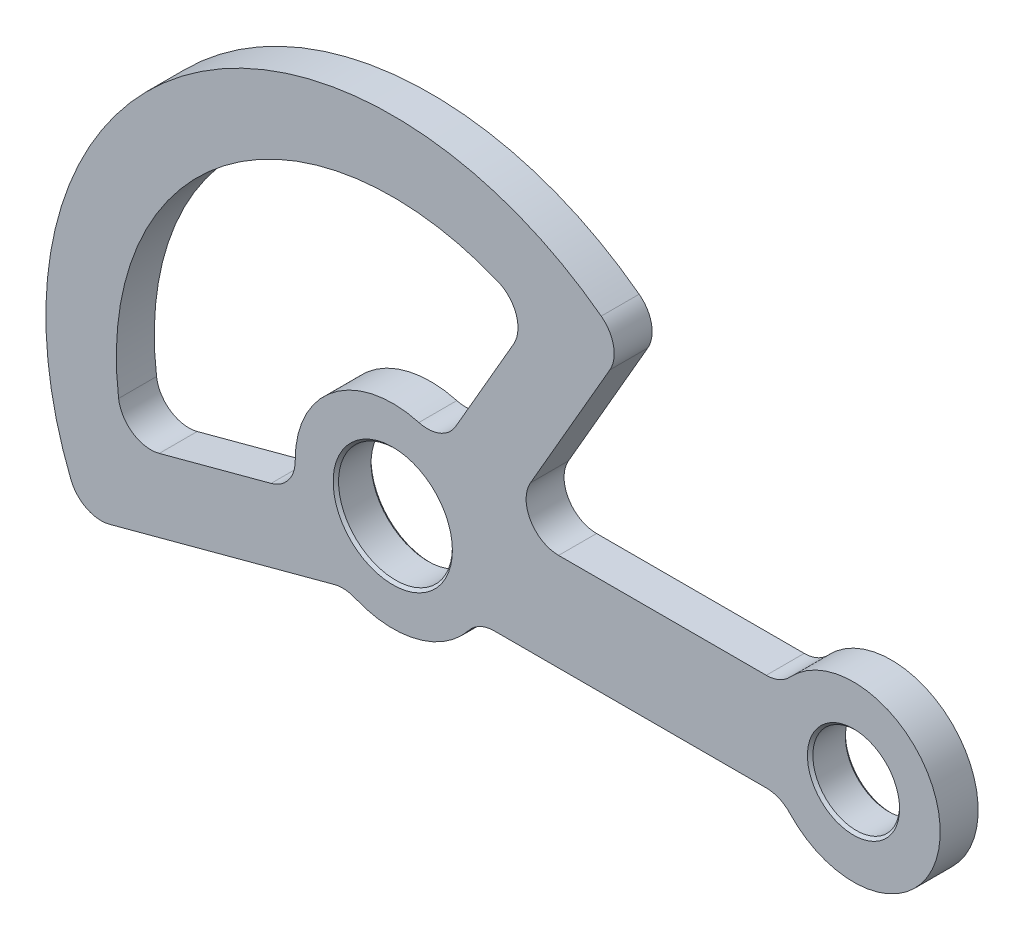
ISO-10303-21;
HEADER;
FILE_DESCRIPTION(('STEP AP214'),'2;1');
FILE_NAME('part.step','',(''),(''),'','','');
FILE_SCHEMA(('AUTOMOTIVE_DESIGN { 1 0 10303 214 1 1 1 1 }'));
ENDSEC;
DATA;
#1=APPLICATION_CONTEXT('core data for automotive mechanical design processes');
#2=APPLICATION_PROTOCOL_DEFINITION('international standard','automotive_design',2000,#1);
#3=PRODUCT_CONTEXT('',#1,'mechanical');
#4=PRODUCT('Part','Part','',(#3));
#5=PRODUCT_RELATED_PRODUCT_CATEGORY('part','',(#4));
#6=PRODUCT_DEFINITION_FORMATION('','',#4);
#7=PRODUCT_DEFINITION_CONTEXT('part definition',#1,'design');
#8=PRODUCT_DEFINITION('design','',#6,#7);
#9=PRODUCT_DEFINITION_SHAPE('','',#8);
#10=(LENGTH_UNIT() NAMED_UNIT(*) SI_UNIT(.MILLI.,.METRE.));
#11=(NAMED_UNIT(*) PLANE_ANGLE_UNIT() SI_UNIT($,.RADIAN.));
#12=(NAMED_UNIT(*) SI_UNIT($,.STERADIAN.) SOLID_ANGLE_UNIT());
#13=UNCERTAINTY_MEASURE_WITH_UNIT(LENGTH_MEASURE(1.E-05),#10,'distance_accuracy_value','');
#14=(GEOMETRIC_REPRESENTATION_CONTEXT(3) GLOBAL_UNCERTAINTY_ASSIGNED_CONTEXT((#13)) GLOBAL_UNIT_ASSIGNED_CONTEXT((#10,
#11,#12)) REPRESENTATION_CONTEXT('',''));
#15=CARTESIAN_POINT('',(0.,0.,0.));
#16=DIRECTION('',(0.,0.,1.));
#17=DIRECTION('',(1.,0.,0.));
#18=AXIS2_PLACEMENT_3D('',#15,#16,#17);
#19=CARTESIAN_POINT('',(85.,0.,3.5));
#20=DIRECTION('',(0.,0.,1.));
#21=DIRECTION('',(1.,0.,0.));
#22=AXIS2_PLACEMENT_3D('',#19,#20,#21);
#23=PLANE('',#22);
#24=CARTESIAN_POINT('',(85.,0.,3.5));
#25=DIRECTION('',(0.,0.,1.));
#26=DIRECTION('',(1.,0.,0.));
#27=AXIS2_PLACEMENT_3D('',#24,#25,#26);
#28=CIRCLE('',#27,8.50000000000004);
#29=CARTESIAN_POINT('',(93.5,0.,3.5));
#30=VERTEX_POINT('',#29);
#31=EDGE_CURVE('E329',#30,#30,#28,.F.);
#32=ORIENTED_EDGE('',*,*,#31,.T.);
#33=EDGE_LOOP('',(#32));
#34=FACE_BOUND('',#33,.T.);
#35=CARTESIAN_POINT('',(0.,0.,3.5));
#36=DIRECTION('',(0.,0.,1.));
#37=DIRECTION('',(1.,0.,0.));
#38=AXIS2_PLACEMENT_3D('',#35,#36,#37);
#39=CIRCLE('',#38,11.);
#40=CARTESIAN_POINT('',(11.,0.,3.5));
#41=VERTEX_POINT('',#40);
#42=EDGE_CURVE('E330',#41,#41,#39,.F.);
#43=ORIENTED_EDGE('',*,*,#42,.T.);
#44=EDGE_LOOP('',(#43));
#45=FACE_BOUND('',#44,.T.);
#46=CARTESIAN_POINT('',(0.,0.,3.5));
#47=DIRECTION('',(0.,0.,1.));
#48=DIRECTION('',(-1.,0.,0.));
#49=AXIS2_PLACEMENT_3D('',#46,#47,#48);
#50=CIRCLE('',#49,64.);
#51=CARTESIAN_POINT('',(38.4553888744394,51.1584114932788,3.5));
#52=VERTEX_POINT('',#51);
#53=CARTESIAN_POINT('',(-59.36821792081,-23.9042820621581,3.5));
#54=VERTEX_POINT('',#53);
#55=EDGE_CURVE('E511',#52,#54,#50,.T.);
#56=ORIENTED_EDGE('',*,*,#55,.T.);
#57=CARTESIAN_POINT('',(-53.8024474907341,-21.6632556188308,3.5));
#58=DIRECTION('',(0.,0.,1.));
#59=DIRECTION('',(1.,0.,0.));
#60=AXIS2_PLACEMENT_3D('',#57,#58,#59);
#61=CIRCLE('',#60,6.);
#62=CARTESIAN_POINT('',(-52.249533220119,-27.4588105765652,3.5));
#63=VERTEX_POINT('',#62);
#64=EDGE_CURVE('E242',#54,#63,#61,.T.);
#65=ORIENTED_EDGE('',*,*,#64,.T.);
#66=DIRECTION('',(0.965925826289069,0.258819045102517,0.));
#67=VECTOR('',#66,1.);
#68=CARTESIAN_POINT('',(-8.66103197007008,-15.7793068673318,3.5));
#69=LINE('',#68,#67);
#70=CARTESIAN_POINT('',(-10.7986052500327,-16.3520679014601,3.5));
#71=VERTEX_POINT('',#70);
#72=EDGE_CURVE('E213',#63,#71,#69,.T.);
#73=ORIENTED_EDGE('',*,*,#72,.T.);
#74=CARTESIAN_POINT('',(-9.2456909794176,-22.1476228591945,3.5));
#75=DIRECTION('',(0.,0.,1.));
#76=DIRECTION('',(1.,0.,0.));
#77=AXIS2_PLACEMENT_3D('',#74,#75,#76);
#78=CIRCLE('',#77,6.);
#79=CARTESIAN_POINT('',(-6.9342682345632,-16.6107171443959,3.5));
#80=VERTEX_POINT('',#79);
#81=EDGE_CURVE('E305',#71,#80,#78,.F.);
#82=ORIENTED_EDGE('',*,*,#81,.T.);
#83=CARTESIAN_POINT('',(0.,0.,3.5));
#84=DIRECTION('',(0.,0.,1.));
#85=DIRECTION('',(1.,0.,0.));
#86=AXIS2_PLACEMENT_3D('',#83,#84,#85);
#87=CIRCLE('',#86,18.);
#88=CARTESIAN_POINT('',(14.0512454963964,-11.25,3.5));
#89=VERTEX_POINT('',#88);
#90=EDGE_CURVE('E519',#80,#89,#87,.T.);
#91=ORIENTED_EDGE('',*,*,#90,.T.);
#92=CARTESIAN_POINT('',(18.7349939951952,-15.,3.5));
#93=DIRECTION('',(0.,0.,1.));
#94=DIRECTION('',(1.,0.,0.));
#95=AXIS2_PLACEMENT_3D('',#92,#93,#94);
#96=CIRCLE('',#95,6.);
#97=CARTESIAN_POINT('',(18.7349939951952,-9.,3.5));
#98=VERTEX_POINT('',#97);
#99=EDGE_CURVE('E307',#89,#98,#96,.F.);
#100=ORIENTED_EDGE('',*,*,#99,.T.);
#101=DIRECTION('',(1.,0.,0.));
#102=VECTOR('',#101,1.);
#103=CARTESIAN_POINT('',(15.5884572681199,-9.,3.5));
#104=LINE('',#103,#102);
#105=CARTESIAN_POINT('',(68.9065230605689,-9.,3.5));
#106=VERTEX_POINT('',#105);
#107=EDGE_CURVE('E235',#98,#106,#104,.T.);
#108=ORIENTED_EDGE('',*,*,#107,.T.);
#109=CARTESIAN_POINT('',(68.9065230605689,-15.,3.5));
#110=DIRECTION('',(0.,0.,1.));
#111=DIRECTION('',(1.,0.,0.));
#112=AXIS2_PLACEMENT_3D('',#109,#110,#111);
#113=CIRCLE('',#112,6.);
#114=CARTESIAN_POINT('',(73.2956531349592,-10.9090909090909,3.5));
#115=VERTEX_POINT('',#114);
#116=EDGE_CURVE('E313',#106,#115,#113,.F.);
#117=ORIENTED_EDGE('',*,*,#116,.T.);
#118=CARTESIAN_POINT('',(85.,0.,3.5));
#119=DIRECTION('',(0.,0.,1.));
#120=DIRECTION('',(1.,0.,0.));
#121=AXIS2_PLACEMENT_3D('',#118,#119,#120);
#122=CIRCLE('',#121,16.);
#123=CARTESIAN_POINT('',(73.2956531349592,10.9090909090909,3.5));
#124=VERTEX_POINT('',#123);
#125=EDGE_CURVE('E234',#115,#124,#122,.T.);
#126=ORIENTED_EDGE('',*,*,#125,.T.);
#127=CARTESIAN_POINT('',(68.9065230605689,15.,3.5));
#128=DIRECTION('',(0.,0.,1.));
#129=DIRECTION('',(1.,0.,0.));
#130=AXIS2_PLACEMENT_3D('',#127,#128,#129);
#131=CIRCLE('',#130,6.);
#132=CARTESIAN_POINT('',(68.9065230605689,9.,3.5));
#133=VERTEX_POINT('',#132);
#134=EDGE_CURVE('E312',#124,#133,#131,.F.);
#135=ORIENTED_EDGE('',*,*,#134,.T.);
#136=DIRECTION('',(-1.,0.,0.));
#137=VECTOR('',#136,1.);
#138=CARTESIAN_POINT('',(20.2072594216369,9.,3.5));
#139=LINE('',#138,#137);
#140=CARTESIAN_POINT('',(30.5995642670502,9.,3.5));
#141=VERTEX_POINT('',#140);
#142=EDGE_CURVE('E509',#133,#141,#139,.T.);
#143=ORIENTED_EDGE('',*,*,#142,.T.);
#144=CARTESIAN_POINT('',(30.5995642670502,15.,3.5));
#145=DIRECTION('',(0.,0.,1.));
#146=DIRECTION('',(1.,0.,0.));
#147=AXIS2_PLACEMENT_3D('',#144,#145,#146);
#148=CIRCLE('',#147,6.);
#149=CARTESIAN_POINT('',(25.4034118443436,18.,3.5));
#150=VERTEX_POINT('',#149);
#151=EDGE_CURVE('E317',#141,#150,#148,.F.);
#152=ORIENTED_EDGE('',*,*,#151,.T.);
#153=DIRECTION('',(0.500000000000001,0.866025403784438,0.));
#154=VECTOR('',#153,1.);
#155=CARTESIAN_POINT('',(20.2072594216369,9.,3.5));
#156=LINE('',#155,#154);
#157=CARTESIAN_POINT('',(40.0463485901673,43.3623104157839,3.5));
#158=VERTEX_POINT('',#157);
#159=EDGE_CURVE('E508',#150,#158,#156,.T.);
#160=ORIENTED_EDGE('',*,*,#159,.T.);
#161=CARTESIAN_POINT('',(34.8501961674607,46.3623104157839,3.5));
#162=DIRECTION('',(0.,0.,1.));
#163=DIRECTION('',(1.,0.,0.));
#164=AXIS2_PLACEMENT_3D('',#161,#162,#163);
#165=CIRCLE('',#164,6.);
#166=EDGE_CURVE('E239',#158,#52,#165,.T.);
#167=ORIENTED_EDGE('',*,*,#166,.T.);
#168=EDGE_LOOP('',(#56,#65,#73,#82,#91,#100,#108,#117,#126,#135,#143,#152,#160,#167));
#169=FACE_BOUND('',#168,.T.);
#170=DIRECTION('',(0.500000000000001,0.866025403784438,0.));
#171=VECTOR('',#170,1.);
#172=CARTESIAN_POINT('',(9.00000000000003,15.5884572681199,3.5));
#173=LINE('',#172,#171);
#174=CARTESIAN_POINT('',(11.6189500386223,20.1246117974981,3.5));
#175=VERTEX_POINT('',#174);
#176=CARTESIAN_POINT('',(22.2991031209778,38.6231795687512,3.5));
#177=VERTEX_POINT('',#176);
#178=EDGE_CURVE('E556',#175,#177,#173,.T.);
#179=ORIENTED_EDGE('',*,*,#178,.F.);
#180=CARTESIAN_POINT('',(6.42279761591566,23.1246117974981,3.5));
#181=DIRECTION('',(0.,0.,1.));
#182=DIRECTION('',(1.,0.,0.));
#183=AXIS2_PLACEMENT_3D('',#180,#181,#182);
#184=CIRCLE('',#183,6.);
#185=CARTESIAN_POINT('',(4.81709821193674,17.3434588481236,3.5));
#186=VERTEX_POINT('',#185);
#187=EDGE_CURVE('E298',#175,#186,#184,.F.);
#188=ORIENTED_EDGE('',*,*,#187,.T.);
#189=CARTESIAN_POINT('',(0.,0.,3.5));
#190=DIRECTION('',(0.,0.,-1.));
#191=DIRECTION('',(1.,0.,0.));
#192=AXIS2_PLACEMENT_3D('',#189,#190,#191);
#193=CIRCLE('',#192,18.);
#194=CARTESIAN_POINT('',(-17.9992515779627,-0.16414211283447,3.5));
#195=VERTEX_POINT('',#194);
#196=EDGE_CURVE('E495',#195,#186,#193,.T.);
#197=ORIENTED_EDGE('',*,*,#196,.F.);
#198=CARTESIAN_POINT('',(-23.9990021039503,-0.21885615044596,3.5));
#199=DIRECTION('',(0.,0.,1.));
#200=DIRECTION('',(1.,0.,0.));
#201=AXIS2_PLACEMENT_3D('',#198,#199,#200);
#202=CIRCLE('',#201,6.);
#203=CARTESIAN_POINT('',(-22.4460878333352,-6.01441110818038,3.5));
#204=VERTEX_POINT('',#203);
#205=EDGE_CURVE('E297',#195,#204,#202,.F.);
#206=ORIENTED_EDGE('',*,*,#205,.T.);
#207=DIRECTION('',(0.965925826289069,0.258819045102517,0.));
#208=VECTOR('',#207,1.);
#209=CARTESIAN_POINT('',(-17.3866648732032,-4.65874281184554,3.5));
#210=LINE('',#209,#208);
#211=CARTESIAN_POINT('',(-43.0785592152712,-11.5428651528283,3.5));
#212=VERTEX_POINT('',#211);
#213=EDGE_CURVE('E528',#212,#204,#210,.T.);
#214=ORIENTED_EDGE('',*,*,#213,.F.);
#215=CARTESIAN_POINT('',(-44.6314734858863,-5.74731019509387,3.5));
#216=DIRECTION('',(0.,0.,1.));
#217=DIRECTION('',(1.,0.,0.));
#218=AXIS2_PLACEMENT_3D('',#215,#216,#217);
#219=CIRCLE('',#218,6.);
#220=CARTESIAN_POINT('',(-50.5823366173378,-6.51361822110638,3.5));
#221=VERTEX_POINT('',#220);
#222=EDGE_CURVE('E60',#212,#221,#219,.F.);
#223=ORIENTED_EDGE('',*,*,#222,.T.);
#224=CARTESIAN_POINT('',(0.,0.,3.5));
#225=DIRECTION('',(0.,0.,1.));
#226=DIRECTION('',(-1.,0.,0.));
#227=AXIS2_PLACEMENT_3D('',#224,#225,#226);
#228=CIRCLE('',#227,51.);
#229=CARTESIAN_POINT('',(19.3833441247073,47.1729368445847,3.5));
#230=VERTEX_POINT('',#229);
#231=EDGE_CURVE('E500',#230,#221,#228,.T.);
#232=ORIENTED_EDGE('',*,*,#231,.F.);
#233=CARTESIAN_POINT('',(17.1029506982712,41.6231795687512,3.5));
#234=DIRECTION('',(0.,0.,1.));
#235=DIRECTION('',(1.,0.,0.));
#236=AXIS2_PLACEMENT_3D('',#233,#234,#235);
#237=CIRCLE('',#236,6.);
#238=EDGE_CURVE('E286',#230,#177,#237,.F.);
#239=ORIENTED_EDGE('',*,*,#238,.T.);
#240=EDGE_LOOP('',(#179,#188,#197,#206,#214,#223,#232,#239));
#241=FACE_BOUND('',#240,.T.);
#242=ADVANCED_FACE('F41',(#34,#45,#169,#241),#23,.T.);
#243=CARTESIAN_POINT('',(85.,0.,-3.5));
#244=DIRECTION('',(0.,0.,1.));
#245=DIRECTION('',(1.,0.,0.));
#246=AXIS2_PLACEMENT_3D('',#243,#244,#245);
#247=PLANE('',#246);
#248=CARTESIAN_POINT('',(85.,0.,-3.5));
#249=DIRECTION('',(0.,0.,1.));
#250=DIRECTION('',(1.,0.,0.));
#251=AXIS2_PLACEMENT_3D('',#248,#249,#250);
#252=CIRCLE('',#251,8.49999999999995);
#253=CARTESIAN_POINT('',(93.5,0.,-3.5));
#254=VERTEX_POINT('',#253);
#255=EDGE_CURVE('E337',#254,#254,#252,.T.);
#256=ORIENTED_EDGE('',*,*,#255,.T.);
#257=EDGE_LOOP('',(#256));
#258=FACE_BOUND('',#257,.T.);
#259=CARTESIAN_POINT('',(0.,0.,-3.5));
#260=DIRECTION('',(0.,0.,1.));
#261=DIRECTION('',(1.,0.,0.));
#262=AXIS2_PLACEMENT_3D('',#259,#260,#261);
#263=CIRCLE('',#262,11.0000000000001);
#264=CARTESIAN_POINT('',(11.0000000000001,0.,-3.5));
#265=VERTEX_POINT('',#264);
#266=EDGE_CURVE('E334',#265,#265,#263,.T.);
#267=ORIENTED_EDGE('',*,*,#266,.T.);
#268=EDGE_LOOP('',(#267));
#269=FACE_BOUND('',#268,.T.);
#270=DIRECTION('',(0.965925826289069,0.258819045102517,0.));
#271=VECTOR('',#270,1.);
#272=CARTESIAN_POINT('',(-8.66103197007008,-15.7793068673318,-3.5));
#273=LINE('',#272,#271);
#274=CARTESIAN_POINT('',(-52.249533220119,-27.4588105765652,-3.5));
#275=VERTEX_POINT('',#274);
#276=CARTESIAN_POINT('',(-10.7986052500327,-16.3520679014601,-3.5));
#277=VERTEX_POINT('',#276);
#278=EDGE_CURVE('E209',#275,#277,#273,.T.);
#279=ORIENTED_EDGE('',*,*,#278,.F.);
#280=CARTESIAN_POINT('',(-53.8024474907341,-21.6632556188308,-3.5));
#281=DIRECTION('',(0.,0.,1.));
#282=DIRECTION('',(1.,0.,0.));
#283=AXIS2_PLACEMENT_3D('',#280,#281,#282);
#284=CIRCLE('',#283,6.);
#285=CARTESIAN_POINT('',(-59.36821792081,-23.9042820621581,-3.5));
#286=VERTEX_POINT('',#285);
#287=EDGE_CURVE('E195',#275,#286,#284,.F.);
#288=ORIENTED_EDGE('',*,*,#287,.T.);
#289=CARTESIAN_POINT('',(0.,0.,-3.5));
#290=DIRECTION('',(0.,0.,1.));
#291=DIRECTION('',(-1.,0.,0.));
#292=AXIS2_PLACEMENT_3D('',#289,#290,#291);
#293=CIRCLE('',#292,64.);
#294=CARTESIAN_POINT('',(38.4553888744394,51.1584114932788,-3.5));
#295=VERTEX_POINT('',#294);
#296=EDGE_CURVE('E222',#295,#286,#293,.T.);
#297=ORIENTED_EDGE('',*,*,#296,.F.);
#298=CARTESIAN_POINT('',(34.8501961674607,46.3623104157839,-3.5));
#299=DIRECTION('',(0.,0.,1.));
#300=DIRECTION('',(1.,0.,0.));
#301=AXIS2_PLACEMENT_3D('',#298,#299,#300);
#302=CIRCLE('',#301,6.);
#303=CARTESIAN_POINT('',(40.0463485901673,43.3623104157839,-3.5));
#304=VERTEX_POINT('',#303);
#305=EDGE_CURVE('E204',#295,#304,#302,.F.);
#306=ORIENTED_EDGE('',*,*,#305,.T.);
#307=DIRECTION('',(0.500000000000001,0.866025403784438,0.));
#308=VECTOR('',#307,1.);
#309=CARTESIAN_POINT('',(20.2072594216369,9.,-3.5));
#310=LINE('',#309,#308);
#311=CARTESIAN_POINT('',(25.4034118443436,18.,-3.5));
#312=VERTEX_POINT('',#311);
#313=EDGE_CURVE('E227',#312,#304,#310,.T.);
#314=ORIENTED_EDGE('',*,*,#313,.F.);
#315=CARTESIAN_POINT('',(30.5995642670502,15.,-3.5));
#316=DIRECTION('',(0.,0.,1.));
#317=DIRECTION('',(1.,0.,0.));
#318=AXIS2_PLACEMENT_3D('',#315,#316,#317);
#319=CIRCLE('',#318,6.);
#320=CARTESIAN_POINT('',(30.5995642670502,9.,-3.5));
#321=VERTEX_POINT('',#320);
#322=EDGE_CURVE('E320',#312,#321,#319,.T.);
#323=ORIENTED_EDGE('',*,*,#322,.T.);
#324=DIRECTION('',(-1.,0.,0.));
#325=VECTOR('',#324,1.);
#326=CARTESIAN_POINT('',(20.2072594216369,9.,-3.5));
#327=LINE('',#326,#325);
#328=CARTESIAN_POINT('',(68.9065230605689,9.,-3.5));
#329=VERTEX_POINT('',#328);
#330=EDGE_CURVE('E523',#329,#321,#327,.T.);
#331=ORIENTED_EDGE('',*,*,#330,.F.);
#332=CARTESIAN_POINT('',(68.9065230605689,15.,-3.5));
#333=DIRECTION('',(0.,0.,1.));
#334=DIRECTION('',(1.,0.,0.));
#335=AXIS2_PLACEMENT_3D('',#332,#333,#334);
#336=CIRCLE('',#335,6.);
#337=CARTESIAN_POINT('',(73.2956531349592,10.9090909090909,-3.5));
#338=VERTEX_POINT('',#337);
#339=EDGE_CURVE('E311',#329,#338,#336,.T.);
#340=ORIENTED_EDGE('',*,*,#339,.T.);
#341=CARTESIAN_POINT('',(85.,0.,-3.5));
#342=DIRECTION('',(0.,0.,1.));
#343=DIRECTION('',(1.,0.,0.));
#344=AXIS2_PLACEMENT_3D('',#341,#342,#343);
#345=CIRCLE('',#344,16.);
#346=CARTESIAN_POINT('',(73.2956531349592,-10.9090909090909,-3.5));
#347=VERTEX_POINT('',#346);
#348=EDGE_CURVE('E524',#347,#338,#345,.T.);
#349=ORIENTED_EDGE('',*,*,#348,.F.);
#350=CARTESIAN_POINT('',(68.9065230605689,-15.,-3.5));
#351=DIRECTION('',(0.,0.,1.));
#352=DIRECTION('',(1.,0.,0.));
#353=AXIS2_PLACEMENT_3D('',#350,#351,#352);
#354=CIRCLE('',#353,6.);
#355=CARTESIAN_POINT('',(68.9065230605689,-9.,-3.5));
#356=VERTEX_POINT('',#355);
#357=EDGE_CURVE('E310',#347,#356,#354,.T.);
#358=ORIENTED_EDGE('',*,*,#357,.T.);
#359=DIRECTION('',(1.,0.,0.));
#360=VECTOR('',#359,1.);
#361=CARTESIAN_POINT('',(15.5884572681199,-9.,-3.5));
#362=LINE('',#361,#360);
#363=CARTESIAN_POINT('',(18.7349939951952,-9.,-3.5));
#364=VERTEX_POINT('',#363);
#365=EDGE_CURVE('E221',#364,#356,#362,.T.);
#366=ORIENTED_EDGE('',*,*,#365,.F.);
#367=CARTESIAN_POINT('',(18.7349939951952,-15.,-3.5));
#368=DIRECTION('',(0.,0.,1.));
#369=DIRECTION('',(1.,0.,0.));
#370=AXIS2_PLACEMENT_3D('',#367,#368,#369);
#371=CIRCLE('',#370,6.);
#372=CARTESIAN_POINT('',(14.0512454963964,-11.25,-3.5));
#373=VERTEX_POINT('',#372);
#374=EDGE_CURVE('E303',#364,#373,#371,.T.);
#375=ORIENTED_EDGE('',*,*,#374,.T.);
#376=CARTESIAN_POINT('',(0.,0.,-3.5));
#377=DIRECTION('',(0.,0.,1.));
#378=DIRECTION('',(1.,0.,0.));
#379=AXIS2_PLACEMENT_3D('',#376,#377,#378);
#380=CIRCLE('',#379,18.);
#381=CARTESIAN_POINT('',(-6.9342682345632,-16.6107171443959,-3.5));
#382=VERTEX_POINT('',#381);
#383=EDGE_CURVE('E219',#382,#373,#380,.T.);
#384=ORIENTED_EDGE('',*,*,#383,.F.);
#385=CARTESIAN_POINT('',(-9.2456909794176,-22.1476228591945,-3.5));
#386=DIRECTION('',(0.,0.,1.));
#387=DIRECTION('',(1.,0.,0.));
#388=AXIS2_PLACEMENT_3D('',#385,#386,#387);
#389=CIRCLE('',#388,6.);
#390=EDGE_CURVE('E218',#382,#277,#389,.T.);
#391=ORIENTED_EDGE('',*,*,#390,.T.);
#392=EDGE_LOOP('',(#279,#288,#297,#306,#314,#323,#331,#340,#349,#358,#366,#375,#384,#391));
#393=FACE_BOUND('',#392,.T.);
#394=DIRECTION('',(0.965925826289069,0.258819045102517,0.));
#395=VECTOR('',#394,1.);
#396=CARTESIAN_POINT('',(-17.3866648732032,-4.65874281184554,-3.5));
#397=LINE('',#396,#395);
#398=CARTESIAN_POINT('',(-43.0785592152712,-11.5428651528283,-3.5));
#399=VERTEX_POINT('',#398);
#400=CARTESIAN_POINT('',(-22.4460878333352,-6.01441110818038,-3.5));
#401=VERTEX_POINT('',#400);
#402=EDGE_CURVE('E488',#399,#401,#397,.T.);
#403=ORIENTED_EDGE('',*,*,#402,.T.);
#404=CARTESIAN_POINT('',(-23.9990021039503,-0.21885615044596,-3.5));
#405=DIRECTION('',(0.,0.,1.));
#406=DIRECTION('',(1.,0.,0.));
#407=AXIS2_PLACEMENT_3D('',#404,#405,#406);
#408=CIRCLE('',#407,6.);
#409=CARTESIAN_POINT('',(-17.9992515779627,-0.16414211283447,-3.5));
#410=VERTEX_POINT('',#409);
#411=EDGE_CURVE('E294',#401,#410,#408,.T.);
#412=ORIENTED_EDGE('',*,*,#411,.T.);
#413=CARTESIAN_POINT('',(0.,0.,-3.5));
#414=DIRECTION('',(0.,0.,-1.));
#415=DIRECTION('',(1.,0.,0.));
#416=AXIS2_PLACEMENT_3D('',#413,#414,#415);
#417=CIRCLE('',#416,18.);
#418=CARTESIAN_POINT('',(4.81709821193674,17.3434588481236,-3.5));
#419=VERTEX_POINT('',#418);
#420=EDGE_CURVE('E502',#410,#419,#417,.T.);
#421=ORIENTED_EDGE('',*,*,#420,.T.);
#422=CARTESIAN_POINT('',(6.42279761591566,23.1246117974981,-3.5));
#423=DIRECTION('',(0.,0.,1.));
#424=DIRECTION('',(1.,0.,0.));
#425=AXIS2_PLACEMENT_3D('',#422,#423,#424);
#426=CIRCLE('',#425,6.);
#427=CARTESIAN_POINT('',(11.6189500386223,20.1246117974981,-3.5));
#428=VERTEX_POINT('',#427);
#429=EDGE_CURVE('E300',#419,#428,#426,.T.);
#430=ORIENTED_EDGE('',*,*,#429,.T.);
#431=DIRECTION('',(0.500000000000001,0.866025403784438,0.));
#432=VECTOR('',#431,1.);
#433=CARTESIAN_POINT('',(9.00000000000003,15.5884572681199,-3.5));
#434=LINE('',#433,#432);
#435=CARTESIAN_POINT('',(22.2991031209778,38.6231795687512,-3.5));
#436=VERTEX_POINT('',#435);
#437=EDGE_CURVE('E496',#428,#436,#434,.T.);
#438=ORIENTED_EDGE('',*,*,#437,.T.);
#439=CARTESIAN_POINT('',(17.1029506982712,41.6231795687512,-3.5));
#440=DIRECTION('',(0.,0.,1.));
#441=DIRECTION('',(1.,0.,0.));
#442=AXIS2_PLACEMENT_3D('',#439,#440,#441);
#443=CIRCLE('',#442,6.);
#444=CARTESIAN_POINT('',(19.3833441247073,47.1729368445847,-3.5));
#445=VERTEX_POINT('',#444);
#446=EDGE_CURVE('E289',#436,#445,#443,.T.);
#447=ORIENTED_EDGE('',*,*,#446,.T.);
#448=CARTESIAN_POINT('',(0.,0.,-3.5));
#449=DIRECTION('',(0.,0.,1.));
#450=DIRECTION('',(-1.,0.,0.));
#451=AXIS2_PLACEMENT_3D('',#448,#449,#450);
#452=CIRCLE('',#451,51.);
#453=CARTESIAN_POINT('',(-50.5823366173378,-6.51361822110638,-3.5));
#454=VERTEX_POINT('',#453);
#455=EDGE_CURVE('E492',#445,#454,#452,.T.);
#456=ORIENTED_EDGE('',*,*,#455,.T.);
#457=CARTESIAN_POINT('',(-44.6314734858863,-5.74731019509387,-3.5));
#458=DIRECTION('',(0.,0.,1.));
#459=DIRECTION('',(1.,0.,0.));
#460=AXIS2_PLACEMENT_3D('',#457,#458,#459);
#461=CIRCLE('',#460,6.);
#462=EDGE_CURVE('E292',#454,#399,#461,.T.);
#463=ORIENTED_EDGE('',*,*,#462,.T.);
#464=EDGE_LOOP('',(#403,#412,#421,#430,#438,#447,#456,#463));
#465=FACE_BOUND('',#464,.T.);
#466=ADVANCED_FACE('F216',(#258,#269,#393,#465),#247,.F.);
#467=CARTESIAN_POINT('',(85.,0.,3.5));
#468=DIRECTION('',(0.,0.,-1.));
#469=DIRECTION('',(-1.,0.,0.));
#470=AXIS2_PLACEMENT_3D('',#467,#468,#469);
#471=CYLINDRICAL_SURFACE('',#470,16.);
#472=ORIENTED_EDGE('',*,*,#125,.F.);
#473=DIRECTION('',(0.,0.,-1.));
#474=VECTOR('',#473,1.);
#475=CARTESIAN_POINT('',(73.2956531349592,-10.9090909090909,3.5));
#476=LINE('',#475,#474);
#477=EDGE_CURVE('E276',#115,#347,#476,.T.);
#478=ORIENTED_EDGE('',*,*,#477,.T.);
#479=ORIENTED_EDGE('',*,*,#348,.T.);
#480=DIRECTION('',(0.,0.,-1.));
#481=VECTOR('',#480,1.);
#482=CARTESIAN_POINT('',(73.2956531349592,10.9090909090909,3.5));
#483=LINE('',#482,#481);
#484=EDGE_CURVE('E280',#338,#124,#483,.F.);
#485=ORIENTED_EDGE('',*,*,#484,.T.);
#486=EDGE_LOOP('',(#472,#478,#479,#485));
#487=FACE_BOUND('',#486,.T.);
#488=ADVANCED_FACE('F356',(#487),#471,.T.);
#489=CARTESIAN_POINT('',(20.2072594216369,9.,3.5));
#490=DIRECTION('',(0.,-1.,0.));
#491=DIRECTION('',(0.,0.,-1.));
#492=AXIS2_PLACEMENT_3D('',#489,#490,#491);
#493=PLANE('',#492);
#494=ORIENTED_EDGE('',*,*,#142,.F.);
#495=DIRECTION('',(0.,0.,1.));
#496=VECTOR('',#495,1.);
#497=CARTESIAN_POINT('',(68.9065230605689,9.,-3.5));
#498=LINE('',#497,#496);
#499=EDGE_CURVE('E281',#133,#329,#498,.F.);
#500=ORIENTED_EDGE('',*,*,#499,.T.);
#501=ORIENTED_EDGE('',*,*,#330,.T.);
#502=DIRECTION('',(0.,0.,-1.));
#503=VECTOR('',#502,1.);
#504=CARTESIAN_POINT('',(30.5995642670502,9.,3.5));
#505=LINE('',#504,#503);
#506=EDGE_CURVE('E284',#321,#141,#505,.F.);
#507=ORIENTED_EDGE('',*,*,#506,.T.);
#508=EDGE_LOOP('',(#494,#500,#501,#507));
#509=FACE_BOUND('',#508,.T.);
#510=ADVANCED_FACE('F383',(#509),#493,.F.);
#511=CARTESIAN_POINT('',(20.2072594216369,9.,3.5));
#512=DIRECTION('',(-0.866025403784438,0.500000000000001,0.));
#513=DIRECTION('',(-0.500000000000001,-0.866025403784438,0.));
#514=AXIS2_PLACEMENT_3D('',#511,#512,#513);
#515=PLANE('',#514);
#516=ORIENTED_EDGE('',*,*,#313,.T.);
#517=DIRECTION('',(0.,0.,-1.));
#518=VECTOR('',#517,1.);
#519=CARTESIAN_POINT('',(40.0463485901673,43.3623104157839,3.5));
#520=LINE('',#519,#518);
#521=EDGE_CURVE('E247',#304,#158,#520,.F.);
#522=ORIENTED_EDGE('',*,*,#521,.T.);
#523=ORIENTED_EDGE('',*,*,#159,.F.);
#524=DIRECTION('',(0.,0.,-1.));
#525=VECTOR('',#524,1.);
#526=CARTESIAN_POINT('',(25.4034118443436,18.,-3.5));
#527=LINE('',#526,#525);
#528=EDGE_CURVE('E245',#150,#312,#527,.T.);
#529=ORIENTED_EDGE('',*,*,#528,.T.);
#530=EDGE_LOOP('',(#516,#522,#523,#529));
#531=FACE_BOUND('',#530,.T.);
#532=ADVANCED_FACE('F379',(#531),#515,.F.);
#533=CARTESIAN_POINT('',(0.,0.,3.5));
#534=DIRECTION('',(0.,0.,-1.));
#535=DIRECTION('',(-1.,0.,0.));
#536=AXIS2_PLACEMENT_3D('',#533,#534,#535);
#537=CYLINDRICAL_SURFACE('',#536,64.);
#538=ORIENTED_EDGE('',*,*,#296,.T.);
#539=DIRECTION('',(0.,0.,-1.));
#540=VECTOR('',#539,1.);
#541=CARTESIAN_POINT('',(-59.36821792081,-23.9042820621581,3.5));
#542=LINE('',#541,#540);
#543=EDGE_CURVE('E196',#286,#54,#542,.F.);
#544=ORIENTED_EDGE('',*,*,#543,.T.);
#545=ORIENTED_EDGE('',*,*,#55,.F.);
#546=DIRECTION('',(0.,0.,-1.));
#547=VECTOR('',#546,1.);
#548=CARTESIAN_POINT('',(38.4553888744394,51.1584114932788,3.5));
#549=LINE('',#548,#547);
#550=EDGE_CURVE('E201',#52,#295,#549,.T.);
#551=ORIENTED_EDGE('',*,*,#550,.T.);
#552=EDGE_LOOP('',(#538,#544,#545,#551));
#553=FACE_BOUND('',#552,.T.);
#554=ADVANCED_FACE('F380',(#553),#537,.T.);
#555=CARTESIAN_POINT('',(-8.66103197007008,-15.7793068673318,3.5));
#556=DIRECTION('',(-0.258819045102517,0.96592582628907,0.));
#557=DIRECTION('',(-0.96592582628907,-0.258819045102517,0.));
#558=AXIS2_PLACEMENT_3D('',#555,#556,#557);
#559=PLANE('',#558);
#560=ORIENTED_EDGE('',*,*,#72,.F.);
#561=DIRECTION('',(0.,0.,-1.));
#562=VECTOR('',#561,1.);
#563=CARTESIAN_POINT('',(-52.249533220119,-27.4588105765652,3.5));
#564=LINE('',#563,#562);
#565=EDGE_CURVE('E197',#63,#275,#564,.T.);
#566=ORIENTED_EDGE('',*,*,#565,.T.);
#567=ORIENTED_EDGE('',*,*,#278,.T.);
#568=DIRECTION('',(0.,0.,1.));
#569=VECTOR('',#568,1.);
#570=CARTESIAN_POINT('',(-10.7986052500327,-16.3520679014601,3.5));
#571=LINE('',#570,#569);
#572=EDGE_CURVE('E212',#277,#71,#571,.T.);
#573=ORIENTED_EDGE('',*,*,#572,.T.);
#574=EDGE_LOOP('',(#560,#566,#567,#573));
#575=FACE_BOUND('',#574,.T.);
#576=ADVANCED_FACE('F207',(#575),#559,.F.);
#577=CARTESIAN_POINT('',(0.,0.,3.5));
#578=DIRECTION('',(0.,0.,-1.));
#579=DIRECTION('',(-1.,0.,0.));
#580=AXIS2_PLACEMENT_3D('',#577,#578,#579);
#581=CYLINDRICAL_SURFACE('',#580,18.);
#582=ORIENTED_EDGE('',*,*,#90,.F.);
#583=DIRECTION('',(0.,0.,-1.));
#584=VECTOR('',#583,1.);
#585=CARTESIAN_POINT('',(-6.9342682345632,-16.6107171443959,3.5));
#586=LINE('',#585,#584);
#587=EDGE_CURVE('E267',#80,#382,#586,.T.);
#588=ORIENTED_EDGE('',*,*,#587,.T.);
#589=ORIENTED_EDGE('',*,*,#383,.T.);
#590=DIRECTION('',(0.,0.,-1.));
#591=VECTOR('',#590,1.);
#592=CARTESIAN_POINT('',(14.0512454963964,-11.25,3.5));
#593=LINE('',#592,#591);
#594=EDGE_CURVE('E270',#373,#89,#593,.F.);
#595=ORIENTED_EDGE('',*,*,#594,.T.);
#596=EDGE_LOOP('',(#582,#588,#589,#595));
#597=FACE_BOUND('',#596,.T.);
#598=ADVANCED_FACE('F367',(#597),#581,.T.);
#599=CARTESIAN_POINT('',(15.5884572681199,-9.,3.5));
#600=DIRECTION('',(0.,1.,0.));
#601=DIRECTION('',(0.,0.,1.));
#602=AXIS2_PLACEMENT_3D('',#599,#600,#601);
#603=PLANE('',#602);
#604=ORIENTED_EDGE('',*,*,#107,.F.);
#605=DIRECTION('',(0.,0.,1.));
#606=VECTOR('',#605,1.);
#607=CARTESIAN_POINT('',(18.7349939951952,-9.,-3.5));
#608=LINE('',#607,#606);
#609=EDGE_CURVE('E273',#98,#364,#608,.F.);
#610=ORIENTED_EDGE('',*,*,#609,.T.);
#611=ORIENTED_EDGE('',*,*,#365,.T.);
#612=DIRECTION('',(0.,0.,1.));
#613=VECTOR('',#612,1.);
#614=CARTESIAN_POINT('',(68.9065230605689,-9.,3.5));
#615=LINE('',#614,#613);
#616=EDGE_CURVE('E275',#356,#106,#615,.T.);
#617=ORIENTED_EDGE('',*,*,#616,.T.);
#618=EDGE_LOOP('',(#604,#610,#611,#617));
#619=FACE_BOUND('',#618,.T.);
#620=ADVANCED_FACE('F370',(#619),#603,.F.);
#621=CARTESIAN_POINT('',(85.,0.,3.5));
#622=DIRECTION('',(0.,0.,-1.));
#623=DIRECTION('',(-1.,0.,0.));
#624=AXIS2_PLACEMENT_3D('',#621,#622,#623);
#625=CYLINDRICAL_SURFACE('',#624,8.);
#626=CARTESIAN_POINT('',(85.,0.,2.99999999999996));
#627=DIRECTION('',(0.,0.,1.));
#628=DIRECTION('',(1.,0.,0.));
#629=AXIS2_PLACEMENT_3D('',#626,#627,#628);
#630=CIRCLE('',#629,8.);
#631=CARTESIAN_POINT('',(93.,0.,2.99999999999996));
#632=VERTEX_POINT('',#631);
#633=EDGE_CURVE('E322',#632,#632,#630,.T.);
#634=ORIENTED_EDGE('',*,*,#633,.T.);
#635=EDGE_LOOP('',(#634));
#636=FACE_BOUND('',#635,.T.);
#637=CARTESIAN_POINT('',(85.,0.,-3.00000000000002));
#638=DIRECTION('',(0.,0.,1.));
#639=DIRECTION('',(1.,0.,0.));
#640=AXIS2_PLACEMENT_3D('',#637,#638,#639);
#641=CIRCLE('',#640,8.);
#642=CARTESIAN_POINT('',(93.,0.,-3.00000000000002));
#643=VERTEX_POINT('',#642);
#644=EDGE_CURVE('E321',#643,#643,#641,.F.);
#645=ORIENTED_EDGE('',*,*,#644,.T.);
#646=EDGE_LOOP('',(#645));
#647=FACE_BOUND('',#646,.T.);
#648=ADVANCED_FACE('F365',(#636,#647),#625,.F.);
#649=CARTESIAN_POINT('',(0.,0.,3.5));
#650=DIRECTION('',(0.,0.,-1.));
#651=DIRECTION('',(-1.,0.,0.));
#652=AXIS2_PLACEMENT_3D('',#649,#650,#651);
#653=CYLINDRICAL_SURFACE('',#652,10.5);
#654=CARTESIAN_POINT('',(0.,0.,-2.99999999999996));
#655=DIRECTION('',(0.,0.,1.));
#656=DIRECTION('',(1.,0.,0.));
#657=AXIS2_PLACEMENT_3D('',#654,#655,#656);
#658=CIRCLE('',#657,10.5);
#659=CARTESIAN_POINT('',(10.5,0.,-2.99999999999996));
#660=VERTEX_POINT('',#659);
#661=EDGE_CURVE('E11',#660,#660,#658,.F.);
#662=ORIENTED_EDGE('',*,*,#661,.T.);
#663=EDGE_LOOP('',(#662));
#664=FACE_BOUND('',#663,.T.);
#665=CARTESIAN_POINT('',(0.,0.,2.99999999999995));
#666=DIRECTION('',(0.,0.,1.));
#667=DIRECTION('',(1.,0.,0.));
#668=AXIS2_PLACEMENT_3D('',#665,#666,#667);
#669=CIRCLE('',#668,10.5);
#670=CARTESIAN_POINT('',(10.5,0.,2.99999999999995));
#671=VERTEX_POINT('',#670);
#672=EDGE_CURVE('E49',#671,#671,#669,.T.);
#673=ORIENTED_EDGE('',*,*,#672,.T.);
#674=EDGE_LOOP('',(#673));
#675=FACE_BOUND('',#674,.T.);
#676=ADVANCED_FACE('F342',(#664,#675),#653,.F.);
#677=CARTESIAN_POINT('',(0.,0.,3.5));
#678=DIRECTION('',(0.,0.,-1.));
#679=DIRECTION('',(-1.,0.,0.));
#680=AXIS2_PLACEMENT_3D('',#677,#678,#679);
#681=CYLINDRICAL_SURFACE('',#680,18.);
#682=ORIENTED_EDGE('',*,*,#420,.F.);
#683=DIRECTION('',(0.,0.,-1.));
#684=VECTOR('',#683,1.);
#685=CARTESIAN_POINT('',(-17.9992515779627,-0.16414211283447,3.5));
#686=LINE('',#685,#684);
#687=EDGE_CURVE('E264',#410,#195,#686,.F.);
#688=ORIENTED_EDGE('',*,*,#687,.T.);
#689=ORIENTED_EDGE('',*,*,#196,.T.);
#690=DIRECTION('',(0.,0.,-1.));
#691=VECTOR('',#690,1.);
#692=CARTESIAN_POINT('',(4.81709821193674,17.3434588481236,3.5));
#693=LINE('',#692,#691);
#694=EDGE_CURVE('E265',#186,#419,#693,.T.);
#695=ORIENTED_EDGE('',*,*,#694,.T.);
#696=EDGE_LOOP('',(#682,#688,#689,#695));
#697=FACE_BOUND('',#696,.T.);
#698=ADVANCED_FACE('F463',(#697),#681,.T.);
#699=CARTESIAN_POINT('',(9.00000000000003,15.5884572681199,3.5));
#700=DIRECTION('',(-0.866025403784438,0.500000000000001,0.));
#701=DIRECTION('',(-0.500000000000001,-0.866025403784438,0.));
#702=AXIS2_PLACEMENT_3D('',#699,#700,#701);
#703=PLANE('',#702);
#704=ORIENTED_EDGE('',*,*,#178,.T.);
#705=DIRECTION('',(0.,0.,1.));
#706=VECTOR('',#705,1.);
#707=CARTESIAN_POINT('',(22.2991031209778,38.6231795687512,-3.5));
#708=LINE('',#707,#706);
#709=EDGE_CURVE('E248',#177,#436,#708,.F.);
#710=ORIENTED_EDGE('',*,*,#709,.T.);
#711=ORIENTED_EDGE('',*,*,#437,.F.);
#712=DIRECTION('',(0.,0.,1.));
#713=VECTOR('',#712,1.);
#714=CARTESIAN_POINT('',(11.6189500386223,20.1246117974981,3.5));
#715=LINE('',#714,#713);
#716=EDGE_CURVE('E250',#428,#175,#715,.T.);
#717=ORIENTED_EDGE('',*,*,#716,.T.);
#718=EDGE_LOOP('',(#704,#710,#711,#717));
#719=FACE_BOUND('',#718,.T.);
#720=ADVANCED_FACE('F472',(#719),#703,.T.);
#721=CARTESIAN_POINT('',(0.,0.,3.5));
#722=DIRECTION('',(0.,0.,-1.));
#723=DIRECTION('',(-1.,0.,0.));
#724=AXIS2_PLACEMENT_3D('',#721,#722,#723);
#725=CYLINDRICAL_SURFACE('',#724,51.);
#726=ORIENTED_EDGE('',*,*,#455,.F.);
#727=DIRECTION('',(0.,0.,-1.));
#728=VECTOR('',#727,1.);
#729=CARTESIAN_POINT('',(19.3833441247073,47.1729368445847,3.5));
#730=LINE('',#729,#728);
#731=EDGE_CURVE('E61',#445,#230,#730,.F.);
#732=ORIENTED_EDGE('',*,*,#731,.T.);
#733=ORIENTED_EDGE('',*,*,#231,.T.);
#734=DIRECTION('',(0.,0.,-1.));
#735=VECTOR('',#734,1.);
#736=CARTESIAN_POINT('',(-50.5823366173378,-6.51361822110638,3.5));
#737=LINE('',#736,#735);
#738=EDGE_CURVE('E251',#221,#454,#737,.T.);
#739=ORIENTED_EDGE('',*,*,#738,.T.);
#740=EDGE_LOOP('',(#726,#732,#733,#739));
#741=FACE_BOUND('',#740,.T.);
#742=ADVANCED_FACE('F476',(#741),#725,.F.);
#743=CARTESIAN_POINT('',(-17.3866648732032,-4.65874281184554,3.5));
#744=DIRECTION('',(-0.258819045102517,0.965925826289069,0.));
#745=DIRECTION('',(-0.965925826289069,-0.258819045102517,0.));
#746=AXIS2_PLACEMENT_3D('',#743,#744,#745);
#747=PLANE('',#746);
#748=ORIENTED_EDGE('',*,*,#402,.F.);
#749=DIRECTION('',(0.,0.,1.));
#750=VECTOR('',#749,1.);
#751=CARTESIAN_POINT('',(-43.0785592152712,-11.5428651528283,3.5));
#752=LINE('',#751,#750);
#753=EDGE_CURVE('E257',#399,#212,#752,.T.);
#754=ORIENTED_EDGE('',*,*,#753,.T.);
#755=ORIENTED_EDGE('',*,*,#213,.T.);
#756=DIRECTION('',(0.,0.,1.));
#757=VECTOR('',#756,1.);
#758=CARTESIAN_POINT('',(-22.4460878333352,-6.01441110818038,-3.5));
#759=LINE('',#758,#757);
#760=EDGE_CURVE('E260',#204,#401,#759,.F.);
#761=ORIENTED_EDGE('',*,*,#760,.T.);
#762=EDGE_LOOP('',(#748,#754,#755,#761));
#763=FACE_BOUND('',#762,.T.);
#764=ADVANCED_FACE('F393',(#763),#747,.T.);
#765=CARTESIAN_POINT('',(-53.8024474907341,-21.6632556188308,3.5));
#766=DIRECTION('',(0.,0.,-1.));
#767=DIRECTION('',(-1.,0.,0.));
#768=AXIS2_PLACEMENT_3D('',#765,#766,#767);
#769=CYLINDRICAL_SURFACE('',#768,6.);
#770=ORIENTED_EDGE('',*,*,#64,.F.);
#771=ORIENTED_EDGE('',*,*,#543,.F.);
#772=ORIENTED_EDGE('',*,*,#287,.F.);
#773=ORIENTED_EDGE('',*,*,#565,.F.);
#774=EDGE_LOOP('',(#770,#771,#772,#773));
#775=FACE_BOUND('',#774,.T.);
#776=ADVANCED_FACE('F198',(#775),#769,.T.);
#777=CARTESIAN_POINT('',(34.8501961674607,46.3623104157839,3.5));
#778=DIRECTION('',(0.,0.,-1.));
#779=DIRECTION('',(-1.,0.,0.));
#780=AXIS2_PLACEMENT_3D('',#777,#778,#779);
#781=CYLINDRICAL_SURFACE('',#780,6.);
#782=ORIENTED_EDGE('',*,*,#166,.F.);
#783=ORIENTED_EDGE('',*,*,#521,.F.);
#784=ORIENTED_EDGE('',*,*,#305,.F.);
#785=ORIENTED_EDGE('',*,*,#550,.F.);
#786=EDGE_LOOP('',(#782,#783,#784,#785));
#787=FACE_BOUND('',#786,.T.);
#788=ADVANCED_FACE('F391',(#787),#781,.T.);
#789=CARTESIAN_POINT('',(17.1029506982712,41.6231795687512,3.5));
#790=DIRECTION('',(0.,0.,-1.));
#791=DIRECTION('',(-1.,0.,0.));
#792=AXIS2_PLACEMENT_3D('',#789,#790,#791);
#793=CYLINDRICAL_SURFACE('',#792,6.);
#794=ORIENTED_EDGE('',*,*,#238,.F.);
#795=ORIENTED_EDGE('',*,*,#731,.F.);
#796=ORIENTED_EDGE('',*,*,#446,.F.);
#797=ORIENTED_EDGE('',*,*,#709,.F.);
#798=EDGE_LOOP('',(#794,#795,#796,#797));
#799=FACE_BOUND('',#798,.T.);
#800=ADVANCED_FACE('F400',(#799),#793,.F.);
#801=CARTESIAN_POINT('',(-44.6314734858863,-5.74731019509387,3.5));
#802=DIRECTION('',(0.,0.,-1.));
#803=DIRECTION('',(-1.,0.,0.));
#804=AXIS2_PLACEMENT_3D('',#801,#802,#803);
#805=CYLINDRICAL_SURFACE('',#804,6.);
#806=ORIENTED_EDGE('',*,*,#222,.F.);
#807=ORIENTED_EDGE('',*,*,#753,.F.);
#808=ORIENTED_EDGE('',*,*,#462,.F.);
#809=ORIENTED_EDGE('',*,*,#738,.F.);
#810=EDGE_LOOP('',(#806,#807,#808,#809));
#811=FACE_BOUND('',#810,.T.);
#812=ADVANCED_FACE('F405',(#811),#805,.F.);
#813=CARTESIAN_POINT('',(-23.9990021039503,-0.21885615044596,3.5));
#814=DIRECTION('',(0.,0.,-1.));
#815=DIRECTION('',(-1.,0.,0.));
#816=AXIS2_PLACEMENT_3D('',#813,#814,#815);
#817=CYLINDRICAL_SURFACE('',#816,6.);
#818=ORIENTED_EDGE('',*,*,#205,.F.);
#819=ORIENTED_EDGE('',*,*,#687,.F.);
#820=ORIENTED_EDGE('',*,*,#411,.F.);
#821=ORIENTED_EDGE('',*,*,#760,.F.);
#822=EDGE_LOOP('',(#818,#819,#820,#821));
#823=FACE_BOUND('',#822,.T.);
#824=ADVANCED_FACE('F407',(#823),#817,.F.);
#825=CARTESIAN_POINT('',(6.42279761591566,23.1246117974981,3.5));
#826=DIRECTION('',(0.,0.,-1.));
#827=DIRECTION('',(-1.,0.,0.));
#828=AXIS2_PLACEMENT_3D('',#825,#826,#827);
#829=CYLINDRICAL_SURFACE('',#828,6.);
#830=ORIENTED_EDGE('',*,*,#187,.F.);
#831=ORIENTED_EDGE('',*,*,#716,.F.);
#832=ORIENTED_EDGE('',*,*,#429,.F.);
#833=ORIENTED_EDGE('',*,*,#694,.F.);
#834=EDGE_LOOP('',(#830,#831,#832,#833));
#835=FACE_BOUND('',#834,.T.);
#836=ADVANCED_FACE('F408',(#835),#829,.F.);
#837=CARTESIAN_POINT('',(-9.2456909794176,-22.1476228591945,3.5));
#838=DIRECTION('',(0.,0.,-1.));
#839=DIRECTION('',(-1.,0.,0.));
#840=AXIS2_PLACEMENT_3D('',#837,#838,#839);
#841=CYLINDRICAL_SURFACE('',#840,6.);
#842=ORIENTED_EDGE('',*,*,#81,.F.);
#843=ORIENTED_EDGE('',*,*,#572,.F.);
#844=ORIENTED_EDGE('',*,*,#390,.F.);
#845=ORIENTED_EDGE('',*,*,#587,.F.);
#846=EDGE_LOOP('',(#842,#843,#844,#845));
#847=FACE_BOUND('',#846,.T.);
#848=ADVANCED_FACE('F411',(#847),#841,.F.);
#849=CARTESIAN_POINT('',(18.7349939951952,-15.,3.5));
#850=DIRECTION('',(0.,0.,-1.));
#851=DIRECTION('',(-1.,0.,0.));
#852=AXIS2_PLACEMENT_3D('',#849,#850,#851);
#853=CYLINDRICAL_SURFACE('',#852,6.);
#854=ORIENTED_EDGE('',*,*,#99,.F.);
#855=ORIENTED_EDGE('',*,*,#594,.F.);
#856=ORIENTED_EDGE('',*,*,#374,.F.);
#857=ORIENTED_EDGE('',*,*,#609,.F.);
#858=EDGE_LOOP('',(#854,#855,#856,#857));
#859=FACE_BOUND('',#858,.T.);
#860=ADVANCED_FACE('F416',(#859),#853,.F.);
#861=CARTESIAN_POINT('',(68.9065230605689,-15.,3.5));
#862=DIRECTION('',(0.,0.,-1.));
#863=DIRECTION('',(-1.,0.,0.));
#864=AXIS2_PLACEMENT_3D('',#861,#862,#863);
#865=CYLINDRICAL_SURFACE('',#864,6.);
#866=ORIENTED_EDGE('',*,*,#116,.F.);
#867=ORIENTED_EDGE('',*,*,#616,.F.);
#868=ORIENTED_EDGE('',*,*,#357,.F.);
#869=ORIENTED_EDGE('',*,*,#477,.F.);
#870=EDGE_LOOP('',(#866,#867,#868,#869));
#871=FACE_BOUND('',#870,.T.);
#872=ADVANCED_FACE('F425',(#871),#865,.F.);
#873=CARTESIAN_POINT('',(68.9065230605689,15.,3.5));
#874=DIRECTION('',(0.,0.,-1.));
#875=DIRECTION('',(-1.,0.,0.));
#876=AXIS2_PLACEMENT_3D('',#873,#874,#875);
#877=CYLINDRICAL_SURFACE('',#876,6.);
#878=ORIENTED_EDGE('',*,*,#134,.F.);
#879=ORIENTED_EDGE('',*,*,#484,.F.);
#880=ORIENTED_EDGE('',*,*,#339,.F.);
#881=ORIENTED_EDGE('',*,*,#499,.F.);
#882=EDGE_LOOP('',(#878,#879,#880,#881));
#883=FACE_BOUND('',#882,.T.);
#884=ADVANCED_FACE('F426',(#883),#877,.F.);
#885=CARTESIAN_POINT('',(30.5995642670502,15.,3.5));
#886=DIRECTION('',(0.,0.,1.));
#887=DIRECTION('',(1.,0.,0.));
#888=AXIS2_PLACEMENT_3D('',#885,#886,#887);
#889=CYLINDRICAL_SURFACE('',#888,6.);
#890=ORIENTED_EDGE('',*,*,#151,.F.);
#891=ORIENTED_EDGE('',*,*,#506,.F.);
#892=ORIENTED_EDGE('',*,*,#322,.F.);
#893=ORIENTED_EDGE('',*,*,#528,.F.);
#894=EDGE_LOOP('',(#890,#891,#892,#893));
#895=FACE_BOUND('',#894,.T.);
#896=ADVANCED_FACE('F429',(#895),#889,.F.);
#897=CARTESIAN_POINT('',(85.,0.,2.99999999999996));
#898=DIRECTION('',(0.,0.,1.));
#899=DIRECTION('',(1.,0.,0.));
#900=AXIS2_PLACEMENT_3D('',#897,#898,#899);
#901=CONICAL_SURFACE('',#900,8.,0.785398163397448);
#902=ORIENTED_EDGE('',*,*,#31,.F.);
#903=EDGE_LOOP('',(#902));
#904=FACE_BOUND('',#903,.T.);
#905=ORIENTED_EDGE('',*,*,#633,.F.);
#906=EDGE_LOOP('',(#905));
#907=FACE_BOUND('',#906,.T.);
#908=ADVANCED_FACE('F433',(#904,#907),#901,.F.);
#909=CARTESIAN_POINT('',(85.,0.,-3.5));
#910=DIRECTION('',(0.,0.,-1.));
#911=DIRECTION('',(-1.,0.,0.));
#912=AXIS2_PLACEMENT_3D('',#909,#910,#911);
#913=CONICAL_SURFACE('',#912,8.49999999999995,0.785398163397421);
#914=ORIENTED_EDGE('',*,*,#644,.F.);
#915=EDGE_LOOP('',(#914));
#916=FACE_BOUND('',#915,.T.);
#917=ORIENTED_EDGE('',*,*,#255,.F.);
#918=EDGE_LOOP('',(#917));
#919=FACE_BOUND('',#918,.T.);
#920=ADVANCED_FACE('F349',(#916,#919),#913,.F.);
#921=CARTESIAN_POINT('',(0.,0.,-3.5));
#922=DIRECTION('',(0.,0.,-1.));
#923=DIRECTION('',(-1.,0.,0.));
#924=AXIS2_PLACEMENT_3D('',#921,#922,#923);
#925=CONICAL_SURFACE('',#924,11.0000000000001,0.785398163397459);
#926=ORIENTED_EDGE('',*,*,#661,.F.);
#927=EDGE_LOOP('',(#926));
#928=FACE_BOUND('',#927,.T.);
#929=ORIENTED_EDGE('',*,*,#266,.F.);
#930=EDGE_LOOP('',(#929));
#931=FACE_BOUND('',#930,.T.);
#932=ADVANCED_FACE('F341',(#928,#931),#925,.F.);
#933=CARTESIAN_POINT('',(0.,0.,2.99999999999995));
#934=DIRECTION('',(0.,0.,1.));
#935=DIRECTION('',(1.,0.,0.));
#936=AXIS2_PLACEMENT_3D('',#933,#934,#935);
#937=CONICAL_SURFACE('',#936,10.5,0.785398163397438);
#938=ORIENTED_EDGE('',*,*,#42,.F.);
#939=EDGE_LOOP('',(#938));
#940=FACE_BOUND('',#939,.T.);
#941=ORIENTED_EDGE('',*,*,#672,.F.);
#942=EDGE_LOOP('',(#941));
#943=FACE_BOUND('',#942,.T.);
#944=ADVANCED_FACE('F42',(#940,#943),#937,.F.);
#945=CLOSED_SHELL('',(#242,#466,#488,#510,#532,#554,#576,#598,#620,#648,#676,#698,#720,#742,
#764,#776,#788,#800,#812,#824,#836,#848,#860,#872,#884,#896,#908,#920,#932,#944));
#946=MANIFOLD_SOLID_BREP('B2',#945);
#947=ADVANCED_BREP_SHAPE_REPRESENTATION('',(#18,#946),#14);
#948=SHAPE_DEFINITION_REPRESENTATION(#9,#947);
ENDSEC;
END-ISO-10303-21;
